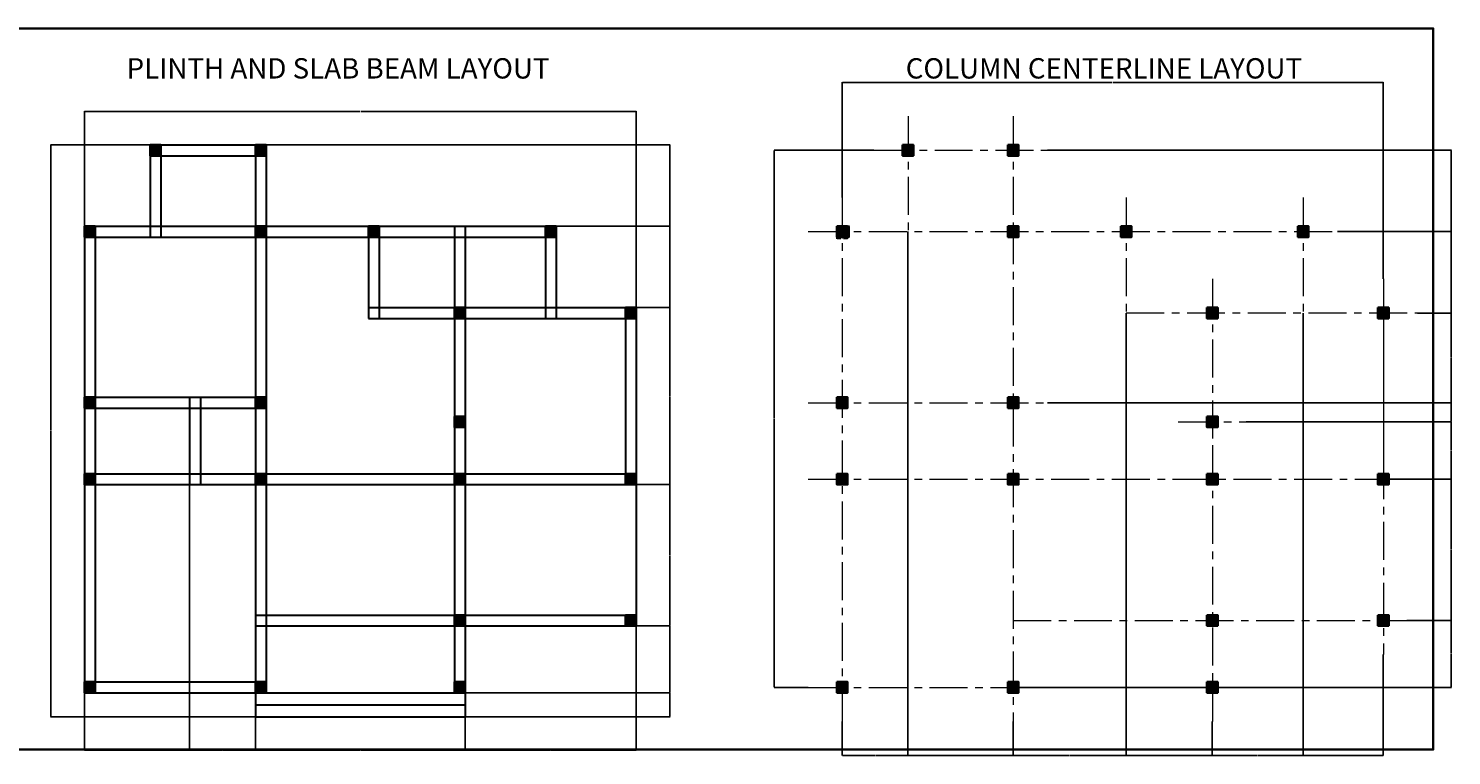
# Model space of a CAD drawing. Units: inches. Extents: x 1332 to 3175, y 1481 to 2088.
# Tile 5 of 5: x 1985 to 3175, y 1481 to 2088. Entities that reach past the tile are written whole.
import ezdxf

# ---------------------------------------------------------------- set-up
doc = ezdxf.new("R2010")
doc.units = ezdxf.units.IN
doc.linetypes.add('CENTER', pattern=[50.8, 31.75, -6.35, 6.35, -6.35])
for name, color, linetype, lineweight in [('A-ANNO-DIMS', 2, 'Continuous', 18), ('A-ANNO-TITL', 6, 'Continuous', 30), ('A-ANNO-TTLB', 7, 'Continuous', 35), ('S-BEAM', 7, 'Continuous', 30), ('S-COLS', 1, 'Continuous', 35), ('S-GRID', 8, 'CENTER', 18)]:
    doc.layers.add(name, color=color, linetype=linetype, lineweight=lineweight)
doc.styles.get("Standard").update_dxf_attribs({"font": 'arial.ttf'})
doc.dimstyles.get("Standard").update_dxf_attribs({"dimtxt": 0.18, "dimasz": 0.18, "dimexe": 0.18, "dimexo": 0.0625, "dimgap": 0.09, "dimtad": 0, "dimtih": 1, "dimtoh": 1, "dimdec": 4, "dimzin": 0, "dimdsep": 46, "dimtxsty": 'Standard', "dimcen": 0.09, "dimadec": 0, "dimazin": 0, "dimtfac": 1, "dimtdec": 4, "dimtofl": 0, "dimtmove": 0, "dimatfit": 3, "dimfxl": 1, "dimtolj": 1, "dimtzin": 0, "dimarcsym": 0})

# ---------------------------------------------------------------- blocks, each defined once
blk = doc.blocks.new('COL-SQUARE-9-STRUCT')
h = blk.add_hatch(color=256)
h.dxf.hatch_style = 1
h.paths.add_polyline_path([(9, 9), (0, 9), (0, 0), (9, 0)])
blk.add_lwpolyline([(0, 9), (9, 9), (9, 0), (0, 0)], close=True)
blk = doc.blocks.new('*D13')
at = {"layer": 'A-ANNO-DIMS', "color": 0, "lineweight": -2, "transparency": 16777216}
for p, q in [((2661, 1914.1), (2661, 1912.6)), ((2661.2, 1912.8), (2664.5, 1912.8)), ((2669.9, 1912.8), (2666.6, 1912.8)), ((2670, 1914.1), (2670, 1912.6))]:
    blk.add_line(p, q, dxfattribs=at)
at = {"layer": 'A-ANNO-DIMS', "color": 0, "transparency": 16777216}
for points in [[(2661.2, 1912.8), (2661.2, 1912.7), (2661, 1912.8)], [(2669.9, 1912.8), (2669.9, 1912.7), (2670, 1912.8)]]:
    blk.add_solid(points, dxfattribs=at)
at = {"layer": 'Defpoints', "color": 0, "transparency": 16777216}
for p in [(2661, 1914.1), (2670, 1914.1), (2670, 1912.8)]:
    blk.add_point(p, dxfattribs=at)
at = {"layer": 'A-ANNO-DIMS', "color": 0, "transparency": 16777216, "insert": (2665.5, 1912.8), "char_height": 0.18, "attachment_point": 5}
blk.add_mtext('\\A1;COLUMN 9 TYP.', dxfattribs=at)
blk = doc.blocks.new('*D14')
at = {"layer": 'A-ANNO-DIMS', "color": 0, "lineweight": -2, "transparency": 16777216}
for p, q in [((2670.1, 1923.1), (2671.6, 1923.1)), ((2671.4, 1922.9), (2671.4, 1918.8)), ((2671.4, 1914.3), (2671.4, 1918.4)), ((2670.1, 1914.1), (2671.6, 1914.1))]:
    blk.add_line(p, q, dxfattribs=at)
at = {"layer": 'A-ANNO-DIMS', "color": 0, "transparency": 16777216}
for points in [[(2671.4, 1922.9), (2671.4, 1922.9), (2671.4, 1923.1)], [(2671.4, 1914.3), (2671.4, 1914.3), (2671.4, 1914.1)]]:
    blk.add_solid(points, dxfattribs=at)
at = {"layer": 'Defpoints', "color": 0, "transparency": 16777216}
for p in [(2670, 1923.1), (2671.4, 1923.1), (2670, 1914.1)]:
    blk.add_point(p, dxfattribs=at)
at = {"layer": 'A-ANNO-DIMS', "color": 0, "transparency": 16777216, "insert": (2671.4, 1918.6), "char_height": 0.18, "attachment_point": 5}
blk.add_mtext('\\A1;9 TYP.', dxfattribs=at)
blk = doc.blocks.new('*D56')
at = {"layer": 'A-ANNO-DIMS', "color": 0, "lineweight": -2, "transparency": 16777216}
for p, q in [((2031.8, 1923.2), (2031.8, 2019.4)), ((2032, 2019.2), (2262.1, 2019.2)), ((2493.1, 2019.2), (2262.9, 2019.2)), ((2493.3, 1855.2), (2493.3, 2019.4))]:
    blk.add_line(p, q, dxfattribs=at)
at = {"layer": 'A-ANNO-DIMS', "color": 0, "transparency": 16777216}
for points in [[(2032, 2019.2), (2032, 2019.2), (2031.8, 2019.2)], [(2493.1, 2019.2), (2493.1, 2019.2), (2493.3, 2019.2)]]:
    blk.add_solid(points, dxfattribs=at)
at = {"layer": 'Defpoints', "color": 0, "transparency": 16777216}
for p in [(2493.3, 2019.2), (2031.8, 1923.1), (2493.3, 1855.1)]:
    blk.add_point(p, dxfattribs=at)
at = {"layer": 'A-ANNO-DIMS', "color": 0, "transparency": 16777216, "insert": (2262.5, 2019.2), "char_height": 0.18, "attachment_point": 5}
blk.add_mtext('\\A1;461.5', dxfattribs=at)
blk = doc.blocks.new('*D57')
at = {"layer": 'A-ANNO-DIMS', "color": 0, "lineweight": -2, "transparency": 16777216}
for p, q in [((2086.7, 1991.1), (2003.5, 1991.1)), ((2003.7, 1990.9), (2003.7, 1752.3)), ((2003.7, 1513.3), (2003.7, 1751.9)), ((2174.7, 1513.1), (2003.5, 1513.1))]:
    blk.add_line(p, q, dxfattribs=at)
at = {"layer": 'A-ANNO-DIMS', "color": 0, "transparency": 16777216}
for points in [[(2003.7, 1990.9), (2003.7, 1990.9), (2003.7, 1991.1)], [(2003.7, 1513.3), (2003.7, 1513.3), (2003.7, 1513.1)]]:
    blk.add_solid(points, dxfattribs=at)
at = {"layer": 'Defpoints', "color": 0, "transparency": 16777216}
for p in [(2003.7, 1991.1), (2086.8, 1991.1), (2174.8, 1513.1)]:
    blk.add_point(p, dxfattribs=at)
at = {"layer": 'A-ANNO-DIMS', "color": 0, "transparency": 16777216, "insert": (2003.7, 1752.1), "char_height": 0.18, "attachment_point": 5}
blk.add_mtext('\\A1;478', dxfattribs=at)
blk = doc.blocks.new('*D58')
at = {"layer": 'A-ANNO-DIMS', "color": 0, "lineweight": -2, "transparency": 16777216}
for p, q in [((2119.8, 1707.1), (2119.8, 1484.8)), ((2031.8, 1533.1), (2031.8, 1484.8)), ((2032, 1485), (2075.6, 1485)), ((2119.6, 1485), (2076, 1485))]:
    blk.add_line(p, q, dxfattribs=at)
at = {"layer": 'A-ANNO-DIMS', "color": 0, "transparency": 16777216}
for points in [[(2032, 1485), (2032, 1485), (2031.8, 1485)], [(2119.6, 1485), (2119.6, 1485), (2119.8, 1485)]]:
    blk.add_solid(points, dxfattribs=at)
at = {"layer": 'Defpoints', "color": 0, "transparency": 16777216}
for p in [(2119.8, 1707.1), (2031.8, 1533.1), (2119.8, 1485)]:
    blk.add_point(p, dxfattribs=at)
at = {"layer": 'A-ANNO-DIMS', "color": 0, "transparency": 16777216, "insert": (2075.8, 1485), "char_height": 0.18, "attachment_point": 5}
blk.add_mtext('\\A1;88', dxfattribs=at)
blk = doc.blocks.new('*D59')
at = {"layer": 'A-ANNO-DIMS', "color": 0, "lineweight": -2, "transparency": 16777216}
for p, q in [((2119.8, 1707.1), (2119.8, 1484.8)), ((2174.8, 1513.1), (2174.8, 1484.8)), ((2120, 1485), (2147.1, 1485)), ((2174.6, 1485), (2147.5, 1485))]:
    blk.add_line(p, q, dxfattribs=at)
at = {"layer": 'A-ANNO-DIMS', "color": 0, "transparency": 16777216}
for points in [[(2120, 1485), (2120, 1485), (2119.8, 1485)], [(2174.6, 1485), (2174.6, 1485), (2174.8, 1485)]]:
    blk.add_solid(points, dxfattribs=at)
at = {"layer": 'Defpoints', "color": 0, "transparency": 16777216}
for p in [(2119.8, 1707.1), (2174.8, 1513.1), (2174.8, 1485)]:
    blk.add_point(p, dxfattribs=at)
at = {"layer": 'A-ANNO-DIMS', "color": 0, "transparency": 16777216, "insert": (2147.3, 1485), "char_height": 0.18, "attachment_point": 5}
blk.add_mtext('\\A1;55', dxfattribs=at)
blk = doc.blocks.new('*D60')
at = {"layer": 'A-ANNO-DIMS', "color": 0, "lineweight": -2, "transparency": 16777216}
for p, q in [((2174.8, 1513.1), (2174.8, 1484.8)), ((2350.3, 1513.1), (2350.3, 1484.8)), ((2175, 1485), (2262.1, 1485)), ((2350.1, 1485), (2262.9, 1485))]:
    blk.add_line(p, q, dxfattribs=at)
at = {"layer": 'A-ANNO-DIMS', "color": 0, "transparency": 16777216}
for points in [[(2175, 1485), (2175, 1485), (2174.8, 1485)], [(2350.1, 1485), (2350.1, 1485), (2350.3, 1485)]]:
    blk.add_solid(points, dxfattribs=at)
at = {"layer": 'Defpoints', "color": 0, "transparency": 16777216}
for p in [(2174.8, 1513.1), (2350.3, 1513.1), (2350.3, 1485)]:
    blk.add_point(p, dxfattribs=at)
at = {"layer": 'A-ANNO-DIMS', "color": 0, "transparency": 16777216, "insert": (2262.5, 1485), "char_height": 0.18, "attachment_point": 5}
blk.add_mtext('\\A1;175.5', dxfattribs=at)
blk = doc.blocks.new('*D61')
at = {"layer": 'A-ANNO-DIMS', "color": 0, "lineweight": -2, "transparency": 16777216}
for p, q in [((2493.3, 1589.1), (2493.3, 1484.8)), ((2350.3, 1513.1), (2350.3, 1484.8)), ((2350.5, 1485), (2421.5, 1485)), ((2493.1, 1485), (2422.1, 1485))]:
    blk.add_line(p, q, dxfattribs=at)
at = {"layer": 'A-ANNO-DIMS', "color": 0, "transparency": 16777216}
for points in [[(2350.5, 1485), (2350.5, 1485), (2350.3, 1485)], [(2493.1, 1485), (2493.1, 1485), (2493.3, 1485)]]:
    blk.add_solid(points, dxfattribs=at)
at = {"layer": 'Defpoints', "color": 0, "transparency": 16777216}
for p in [(2493.3, 1589.1), (2350.3, 1513.1), (2493.3, 1485)]:
    blk.add_point(p, dxfattribs=at)
at = {"layer": 'A-ANNO-DIMS', "color": 0, "transparency": 16777216, "insert": (2421.8, 1485), "char_height": 0.18, "attachment_point": 5}
blk.add_mtext('\\A1;143', dxfattribs=at)
blk = doc.blocks.new('*D62')
at = {"layer": 'A-ANNO-DIMS', "color": 0, "lineweight": -2, "transparency": 16777216}
for p, q in [((2350.3, 1533.1), (2521.6, 1533.1)), ((2521.4, 1532.9), (2521.4, 1523.3)), ((2350.3, 1513.1), (2521.6, 1513.1)), ((2521.4, 1513.3), (2521.4, 1522.9))]:
    blk.add_line(p, q, dxfattribs=at)
at = {"layer": 'A-ANNO-DIMS', "color": 0, "transparency": 16777216}
for points in [[(2521.4, 1532.9), (2521.4, 1532.9), (2521.4, 1533.1)], [(2521.4, 1513.3), (2521.4, 1513.3), (2521.4, 1513.1)]]:
    blk.add_solid(points, dxfattribs=at)
at = {"layer": 'Defpoints', "color": 0, "transparency": 16777216}
for p in [(2350.3, 1533.1), (2521.4, 1533.1), (2350.3, 1513.1)]:
    blk.add_point(p, dxfattribs=at)
at = {"layer": 'A-ANNO-DIMS', "color": 0, "transparency": 16777216, "insert": (2521.4, 1523.1), "char_height": 0.18, "attachment_point": 5}
blk.add_mtext('\\A1;20', dxfattribs=at)
blk = doc.blocks.new('*D63')
at = {"layer": 'A-ANNO-DIMS', "color": 0, "lineweight": -2, "transparency": 16777216}
for p, q in [((2493.3, 1589.1), (2521.6, 1589.1)), ((2521.4, 1588.9), (2521.4, 1561.3)), ((2521.4, 1533.3), (2521.4, 1560.9)), ((2350.3, 1533.1), (2521.6, 1533.1))]:
    blk.add_line(p, q, dxfattribs=at)
at = {"layer": 'A-ANNO-DIMS', "color": 0, "transparency": 16777216}
for points in [[(2521.4, 1588.9), (2521.4, 1588.9), (2521.4, 1589.1)], [(2521.4, 1533.3), (2521.4, 1533.3), (2521.4, 1533.1)]]:
    blk.add_solid(points, dxfattribs=at)
at = {"layer": 'Defpoints', "color": 0, "transparency": 16777216}
for p in [(2493.3, 1589.1), (2521.4, 1589.1), (2350.3, 1533.1)]:
    blk.add_point(p, dxfattribs=at)
at = {"layer": 'A-ANNO-DIMS', "color": 0, "transparency": 16777216, "insert": (2521.4, 1561.1), "char_height": 0.18, "attachment_point": 5}
blk.add_mtext('\\A1;56', dxfattribs=at)
blk = doc.blocks.new('*D64')
at = {"layer": 'A-ANNO-DIMS', "color": 0, "lineweight": -2, "transparency": 16777216}
for p, q in [((2493.3, 1707.1), (2521.6, 1707.1)), ((2521.4, 1706.9), (2521.4, 1648.3)), ((2521.4, 1589.3), (2521.4, 1647.9)), ((2493.3, 1589.1), (2521.6, 1589.1))]:
    blk.add_line(p, q, dxfattribs=at)
at = {"layer": 'A-ANNO-DIMS', "color": 0, "transparency": 16777216}
for points in [[(2521.4, 1706.9), (2521.4, 1706.9), (2521.4, 1707.1)], [(2521.4, 1589.3), (2521.4, 1589.3), (2521.4, 1589.1)]]:
    blk.add_solid(points, dxfattribs=at)
at = {"layer": 'Defpoints', "color": 0, "transparency": 16777216}
for p in [(2493.3, 1707.1), (2521.4, 1707.1), (2493.3, 1589.1)]:
    blk.add_point(p, dxfattribs=at)
at = {"layer": 'A-ANNO-DIMS', "color": 0, "transparency": 16777216, "insert": (2521.4, 1648.1), "char_height": 0.18, "attachment_point": 5}
blk.add_mtext('\\A1;118', dxfattribs=at)
blk = doc.blocks.new('*D65')
at = {"layer": 'A-ANNO-DIMS', "color": 0, "lineweight": -2, "transparency": 16777216}
for p, q in [((2493.3, 1855.1), (2521.6, 1855.1)), ((2521.4, 1854.9), (2521.4, 1781.3)), ((2521.4, 1707.3), (2521.4, 1780.9)), ((2493.3, 1707.1), (2521.6, 1707.1))]:
    blk.add_line(p, q, dxfattribs=at)
at = {"layer": 'A-ANNO-DIMS', "color": 0, "transparency": 16777216}
for points in [[(2521.4, 1854.9), (2521.4, 1854.9), (2521.4, 1855.1)], [(2521.4, 1707.3), (2521.4, 1707.3), (2521.4, 1707.1)]]:
    blk.add_solid(points, dxfattribs=at)
at = {"layer": 'Defpoints', "color": 0, "transparency": 16777216}
for p in [(2493.3, 1855.1), (2521.4, 1855.1), (2493.3, 1707.1)]:
    blk.add_point(p, dxfattribs=at)
at = {"layer": 'A-ANNO-DIMS', "color": 0, "transparency": 16777216, "insert": (2521.4, 1781.1), "char_height": 0.18, "attachment_point": 5}
blk.add_mtext('\\A1;148', dxfattribs=at)
blk = doc.blocks.new('*D66')
at = {"layer": 'A-ANNO-DIMS', "color": 0, "lineweight": -2, "transparency": 16777216}
for p, q in [((2426.3, 1923.1), (2521.6, 1923.1)), ((2521.4, 1922.9), (2521.4, 1889.3)), ((2521.4, 1855.3), (2521.4, 1888.9)), ((2493.3, 1855.1), (2521.6, 1855.1))]:
    blk.add_line(p, q, dxfattribs=at)
at = {"layer": 'A-ANNO-DIMS', "color": 0, "transparency": 16777216}
for points in [[(2521.4, 1922.9), (2521.4, 1922.9), (2521.4, 1923.1)], [(2521.4, 1855.3), (2521.4, 1855.3), (2521.4, 1855.1)]]:
    blk.add_solid(points, dxfattribs=at)
at = {"layer": 'Defpoints', "color": 0, "transparency": 16777216}
for p in [(2426.3, 1923.1), (2521.4, 1923.1), (2493.3, 1855.1)]:
    blk.add_point(p, dxfattribs=at)
at = {"layer": 'A-ANNO-DIMS', "color": 0, "transparency": 16777216, "insert": (2521.4, 1889.1), "char_height": 0.18, "attachment_point": 5}
blk.add_mtext('\\A1;68', dxfattribs=at)
blk = doc.blocks.new('*D67')
at = {"layer": 'A-ANNO-DIMS', "color": 0, "lineweight": -2, "transparency": 16777216}
for p, q in [((2183.8, 1991.1), (2521.6, 1991.1)), ((2521.4, 1990.9), (2521.4, 1957.3)), ((2521.4, 1923.3), (2521.4, 1956.9)), ((2426.3, 1923.1), (2521.6, 1923.1))]:
    blk.add_line(p, q, dxfattribs=at)
at = {"layer": 'A-ANNO-DIMS', "color": 0, "transparency": 16777216}
for points in [[(2521.4, 1990.9), (2521.4, 1990.9), (2521.4, 1991.1)], [(2521.4, 1923.3), (2521.4, 1923.3), (2521.4, 1923.1)]]:
    blk.add_solid(points, dxfattribs=at)
at = {"layer": 'Defpoints', "color": 0, "transparency": 16777216}
for p in [(2183.8, 1991.1), (2521.4, 1991.1), (2426.3, 1923.1)]:
    blk.add_point(p, dxfattribs=at)
at = {"layer": 'A-ANNO-DIMS', "color": 0, "transparency": 16777216, "insert": (2521.4, 1957.1), "char_height": 0.18, "attachment_point": 5}
blk.add_mtext('\\A1;68', dxfattribs=at)
blk = doc.blocks.new('*D68')
at = {"layer": 'A-ANNO-DIMS', "color": 0, "lineweight": -2, "transparency": 16777216}
for p, q in [((2665.5, 1947.2), (2665.5, 2043.6)), ((2665.7, 2043.4), (2891.4, 2043.4)), ((3117.9, 2043.4), (2892.2, 2043.4)), ((3118, 1879.2), (3118, 2043.6))]:
    blk.add_line(p, q, dxfattribs=at)
at = {"layer": 'A-ANNO-DIMS', "color": 0, "transparency": 16777216}
for points in [[(2665.7, 2043.4), (2665.7, 2043.4), (2665.5, 2043.4)], [(3117.9, 2043.4), (3117.9, 2043.4), (3118, 2043.4)]]:
    blk.add_solid(points, dxfattribs=at)
at = {"layer": 'Defpoints', "color": 0, "transparency": 16777216}
for p in [(3118, 2043.4), (2665.5, 1947.1), (3118, 1879.1)]:
    blk.add_point(p, dxfattribs=at)
at = {"layer": 'A-ANNO-DIMS', "color": 0, "transparency": 16777216, "insert": (2891.8, 2043.4), "char_height": 0.18, "attachment_point": 5}
blk.add_mtext('\\A1;452.5', dxfattribs=at)
blk = doc.blocks.new('*D69')
at = {"layer": 'A-ANNO-DIMS', "color": 0, "lineweight": -2, "transparency": 16777216}
for p, q in [((2692, 1986.6), (2608.6, 1986.6)), ((2608.7, 1986.4), (2608.7, 1762.3)), ((2608.7, 1537.8), (2608.7, 1761.9)), ((2637, 1537.6), (2608.6, 1537.6))]:
    blk.add_line(p, q, dxfattribs=at)
at = {"layer": 'A-ANNO-DIMS', "color": 0, "transparency": 16777216}
for points in [[(2608.7, 1986.4), (2608.8, 1986.4), (2608.7, 1986.6)], [(2608.7, 1537.8), (2608.8, 1537.8), (2608.7, 1537.6)]]:
    blk.add_solid(points, dxfattribs=at)
at = {"layer": 'Defpoints', "color": 0, "transparency": 16777216}
for p in [(2608.7, 1986.6), (2692, 1986.6), (2637, 1537.6)]:
    blk.add_point(p, dxfattribs=at)
at = {"layer": 'A-ANNO-DIMS', "color": 0, "transparency": 16777216, "insert": (2608.7, 1762.1), "char_height": 0.18, "attachment_point": 5}
blk.add_mtext('\\A1;449', dxfattribs=at)
blk = doc.blocks.new('*D70')
at = {"layer": 'A-ANNO-DIMS', "color": 0, "lineweight": -2, "transparency": 16777216}
for p, q in [((2720.5, 1918.6), (2720.5, 1480.6)), ((2665.5, 1509.1), (2665.5, 1480.6)), ((2665.7, 1480.8), (2692.8, 1480.8)), ((2720.4, 1480.8), (2693.3, 1480.8))]:
    blk.add_line(p, q, dxfattribs=at)
at = {"layer": 'A-ANNO-DIMS', "color": 0, "transparency": 16777216}
for points in [[(2665.7, 1480.8), (2665.7, 1480.8), (2665.5, 1480.8)], [(2720.4, 1480.8), (2720.4, 1480.8), (2720.5, 1480.8)]]:
    blk.add_solid(points, dxfattribs=at)
at = {"layer": 'Defpoints', "color": 0, "transparency": 16777216}
for p in [(2720.5, 1918.6), (2665.5, 1509.1), (2720.5, 1480.8)]:
    blk.add_point(p, dxfattribs=at)
at = {"layer": 'A-ANNO-DIMS', "color": 0, "transparency": 16777216, "insert": (2693, 1480.8), "char_height": 0.18, "attachment_point": 5}
blk.add_mtext('\\A1;55', dxfattribs=at)
blk = doc.blocks.new('*D71')
at = {"layer": 'A-ANNO-DIMS', "color": 0, "lineweight": -2, "transparency": 16777216}
for p, q in [((2720.5, 1918.6), (2720.5, 1480.6)), ((2808.5, 1509.1), (2808.5, 1480.6)), ((2720.7, 1480.8), (2764.3, 1480.8)), ((2808.4, 1480.8), (2764.8, 1480.8))]:
    blk.add_line(p, q, dxfattribs=at)
at = {"layer": 'A-ANNO-DIMS', "color": 0, "transparency": 16777216}
for points in [[(2720.7, 1480.8), (2720.7, 1480.8), (2720.5, 1480.8)], [(2808.4, 1480.8), (2808.4, 1480.8), (2808.5, 1480.8)]]:
    blk.add_solid(points, dxfattribs=at)
at = {"layer": 'Defpoints', "color": 0, "transparency": 16777216}
for p in [(2720.5, 1918.6), (2808.5, 1509.1), (2808.5, 1480.8)]:
    blk.add_point(p, dxfattribs=at)
at = {"layer": 'A-ANNO-DIMS', "color": 0, "transparency": 16777216, "insert": (2764.5, 1480.8), "char_height": 0.18, "attachment_point": 5}
blk.add_mtext('\\A1;88', dxfattribs=at)
blk = doc.blocks.new('*D72')
at = {"layer": 'A-ANNO-DIMS', "color": 0, "lineweight": -2, "transparency": 16777216}
for p, q in [((2903, 1850.6), (2903, 1480.6)), ((2808.5, 1509.1), (2808.5, 1480.6)), ((2808.7, 1480.8), (2855.5, 1480.8)), ((2902.9, 1480.8), (2856.1, 1480.8))]:
    blk.add_line(p, q, dxfattribs=at)
at = {"layer": 'A-ANNO-DIMS', "color": 0, "transparency": 16777216}
for points in [[(2808.7, 1480.8), (2808.7, 1480.8), (2808.5, 1480.8)], [(2902.9, 1480.8), (2902.9, 1480.8), (2903, 1480.8)]]:
    blk.add_solid(points, dxfattribs=at)
at = {"layer": 'Defpoints', "color": 0, "transparency": 16777216}
for p in [(2903, 1850.6), (2808.5, 1509.1), (2903, 1480.8)]:
    blk.add_point(p, dxfattribs=at)
at = {"layer": 'A-ANNO-DIMS', "color": 0, "transparency": 16777216, "insert": (2855.8, 1480.8), "char_height": 0.18, "attachment_point": 5}
blk.add_mtext('\\A1;94.5', dxfattribs=at)
blk = doc.blocks.new('*D73')
at = {"layer": 'A-ANNO-DIMS', "color": 0, "lineweight": -2, "transparency": 16777216}
for p, q in [((2903, 1850.6), (2903, 1480.6)), ((2975, 1509.1), (2975, 1480.6)), ((2903.2, 1480.8), (2938.8, 1480.8)), ((2974.9, 1480.8), (2939.3, 1480.8))]:
    blk.add_line(p, q, dxfattribs=at)
at = {"layer": 'A-ANNO-DIMS', "color": 0, "transparency": 16777216}
for points in [[(2903.2, 1480.8), (2903.2, 1480.8), (2903, 1480.8)], [(2974.9, 1480.8), (2974.9, 1480.8), (2975, 1480.8)]]:
    blk.add_solid(points, dxfattribs=at)
at = {"layer": 'Defpoints', "color": 0, "transparency": 16777216}
for p in [(2903, 1850.6), (2975, 1509.1), (2975, 1480.8)]:
    blk.add_point(p, dxfattribs=at)
at = {"layer": 'A-ANNO-DIMS', "color": 0, "transparency": 16777216, "insert": (2939, 1480.8), "char_height": 0.18, "attachment_point": 5}
blk.add_mtext('\\A1;72', dxfattribs=at)
blk = doc.blocks.new('*D74')
at = {"layer": 'A-ANNO-DIMS', "color": 0, "lineweight": -2, "transparency": 16777216}
for p, q in [((3051, 1850.6), (3051, 1480.6)), ((2975, 1509.1), (2975, 1480.6)), ((2975.2, 1480.8), (3012.8, 1480.8)), ((3050.9, 1480.8), (3013.3, 1480.8))]:
    blk.add_line(p, q, dxfattribs=at)
at = {"layer": 'A-ANNO-DIMS', "color": 0, "transparency": 16777216}
for points in [[(2975.2, 1480.8), (2975.2, 1480.8), (2975, 1480.8)], [(3050.9, 1480.8), (3050.9, 1480.8), (3051, 1480.8)]]:
    blk.add_solid(points, dxfattribs=at)
at = {"layer": 'Defpoints', "color": 0, "transparency": 16777216}
for p in [(3051, 1850.6), (2975, 1509.1), (3051, 1480.8)]:
    blk.add_point(p, dxfattribs=at)
at = {"layer": 'A-ANNO-DIMS', "color": 0, "transparency": 16777216, "insert": (3013, 1480.8), "char_height": 0.18, "attachment_point": 5}
blk.add_mtext('\\A1;76', dxfattribs=at)
blk = doc.blocks.new('*D75')
at = {"layer": 'A-ANNO-DIMS', "color": 0, "lineweight": -2, "transparency": 16777216}
for p, q in [((3051, 1850.6), (3051, 1480.6)), ((3118, 1565.1), (3118, 1480.6)), ((3051.2, 1480.8), (3084.3, 1480.8)), ((3117.9, 1480.8), (3084.8, 1480.8))]:
    blk.add_line(p, q, dxfattribs=at)
at = {"layer": 'A-ANNO-DIMS', "color": 0, "transparency": 16777216}
for points in [[(3051.2, 1480.8), (3051.2, 1480.8), (3051, 1480.8)], [(3117.9, 1480.8), (3117.9, 1480.8), (3118, 1480.8)]]:
    blk.add_solid(points, dxfattribs=at)
at = {"layer": 'Defpoints', "color": 0, "transparency": 16777216}
for p in [(3051, 1850.6), (3118, 1565.1), (3118, 1480.8)]:
    blk.add_point(p, dxfattribs=at)
at = {"layer": 'A-ANNO-DIMS', "color": 0, "transparency": 16777216, "insert": (3084.5, 1480.8), "char_height": 0.18, "attachment_point": 5}
blk.add_mtext('\\A1;67', dxfattribs=at)
blk = doc.blocks.new('*D76')
at = {"layer": 'A-ANNO-DIMS', "color": 0, "lineweight": -2, "transparency": 16777216}
for p, q in [((3137.6, 1593.6), (3175, 1593.6)), ((3174.8, 1593.4), (3174.8, 1565.8)), ((3174.8, 1537.8), (3174.8, 1565.4)), ((2813.1, 1537.6), (3175, 1537.6))]:
    blk.add_line(p, q, dxfattribs=at)
at = {"layer": 'A-ANNO-DIMS', "color": 0, "transparency": 16777216}
for points in [[(3174.8, 1593.4), (3174.9, 1593.4), (3174.8, 1593.6)], [(3174.8, 1537.8), (3174.9, 1537.8), (3174.8, 1537.6)]]:
    blk.add_solid(points, dxfattribs=at)
at = {"layer": 'Defpoints', "color": 0, "transparency": 16777216}
for p in [(3137.5, 1593.6), (3174.8, 1593.6), (2813, 1537.6)]:
    blk.add_point(p, dxfattribs=at)
at = {"layer": 'A-ANNO-DIMS', "color": 0, "transparency": 16777216, "insert": (3174.8, 1565.6), "char_height": 0.18, "attachment_point": 5}
blk.add_mtext('\\A1;56', dxfattribs=at)
blk = doc.blocks.new('*D77')
at = {"layer": 'A-ANNO-DIMS', "color": 0, "lineweight": -2, "transparency": 16777216}
for p, q in [((3122.6, 1711.6), (3175, 1711.6)), ((3174.8, 1711.4), (3174.8, 1652.8)), ((3174.8, 1593.8), (3174.8, 1652.4)), ((3137.6, 1593.6), (3175, 1593.6))]:
    blk.add_line(p, q, dxfattribs=at)
at = {"layer": 'A-ANNO-DIMS', "color": 0, "transparency": 16777216}
for points in [[(3174.8, 1711.4), (3174.9, 1711.4), (3174.8, 1711.6)], [(3174.8, 1593.8), (3174.9, 1593.8), (3174.8, 1593.6)]]:
    blk.add_solid(points, dxfattribs=at)
at = {"layer": 'Defpoints', "color": 0, "transparency": 16777216}
for p in [(3122.5, 1711.6), (3174.8, 1711.6), (3137.5, 1593.6)]:
    blk.add_point(p, dxfattribs=at)
at = {"layer": 'A-ANNO-DIMS', "color": 0, "transparency": 16777216, "insert": (3174.8, 1652.6), "char_height": 0.18, "attachment_point": 5}
blk.add_mtext('\\A1;118', dxfattribs=at)
blk = doc.blocks.new('*D78')
at = {"layer": 'A-ANNO-DIMS', "color": 0, "lineweight": -2, "transparency": 16777216}
for p, q in [((3003.4, 1759.6), (3175, 1759.6)), ((3174.8, 1759.4), (3174.8, 1735.8)), ((3174.8, 1711.8), (3174.8, 1735.4)), ((3122.6, 1711.6), (3175, 1711.6))]:
    blk.add_line(p, q, dxfattribs=at)
at = {"layer": 'A-ANNO-DIMS', "color": 0, "transparency": 16777216}
for points in [[(3174.8, 1759.4), (3174.9, 1759.4), (3174.8, 1759.6)], [(3174.8, 1711.8), (3174.9, 1711.8), (3174.8, 1711.6)]]:
    blk.add_solid(points, dxfattribs=at)
at = {"layer": 'Defpoints', "color": 0, "transparency": 16777216}
for p in [(3003.3, 1759.6), (3174.8, 1759.6), (3122.5, 1711.6)]:
    blk.add_point(p, dxfattribs=at)
at = {"layer": 'A-ANNO-DIMS', "color": 0, "transparency": 16777216, "insert": (3174.8, 1735.6), "char_height": 0.18, "attachment_point": 5}
blk.add_mtext('\\A1;48', dxfattribs=at)
blk = doc.blocks.new('*D79')
at = {"layer": 'A-ANNO-DIMS', "color": 0, "lineweight": -2, "transparency": 16777216}
for p, q in [((2837.1, 1775.6), (3175, 1775.6)), ((3174.8, 1775.4), (3174.8, 1767.8)), ((3174.8, 1759.8), (3174.8, 1767.4)), ((3003.4, 1759.6), (3175, 1759.6))]:
    blk.add_line(p, q, dxfattribs=at)
at = {"layer": 'A-ANNO-DIMS', "color": 0, "transparency": 16777216}
for points in [[(3174.8, 1775.4), (3174.9, 1775.4), (3174.8, 1775.6)], [(3174.8, 1759.8), (3174.9, 1759.8), (3174.8, 1759.6)]]:
    blk.add_solid(points, dxfattribs=at)
at = {"layer": 'Defpoints', "color": 0, "transparency": 16777216}
for p in [(2837, 1775.6), (3174.8, 1775.6), (3003.3, 1759.6)]:
    blk.add_point(p, dxfattribs=at)
at = {"layer": 'A-ANNO-DIMS', "color": 0, "transparency": 16777216, "insert": (3174.8, 1767.6), "char_height": 0.18, "attachment_point": 5}
blk.add_mtext('\\A1;16', dxfattribs=at)
blk = doc.blocks.new('*D80')
at = {"layer": 'A-ANNO-DIMS', "color": 0, "lineweight": -2, "transparency": 16777216}
for p, q in [((3146.6, 1850.6), (3175, 1850.6)), ((3174.8, 1850.4), (3174.8, 1813.3)), ((3174.8, 1775.8), (3174.8, 1812.9)), ((2837.1, 1775.6), (3175, 1775.6))]:
    blk.add_line(p, q, dxfattribs=at)
at = {"layer": 'A-ANNO-DIMS', "color": 0, "transparency": 16777216}
for points in [[(3174.8, 1850.4), (3174.9, 1850.4), (3174.8, 1850.6)], [(3174.8, 1775.8), (3174.9, 1775.8), (3174.8, 1775.6)]]:
    blk.add_solid(points, dxfattribs=at)
at = {"layer": 'Defpoints', "color": 0, "transparency": 16777216}
for p in [(3146.5, 1850.6), (3174.8, 1850.6), (2837, 1775.6)]:
    blk.add_point(p, dxfattribs=at)
at = {"layer": 'A-ANNO-DIMS', "color": 0, "transparency": 16777216, "insert": (3174.8, 1813.1), "char_height": 0.18, "attachment_point": 5}
blk.add_mtext('\\A1;75', dxfattribs=at)
blk = doc.blocks.new('*D81')
at = {"layer": 'A-ANNO-DIMS', "color": 0, "lineweight": -2, "transparency": 16777216}
for p, q in [((3079.6, 1918.6), (3175, 1918.6)), ((3174.8, 1918.4), (3174.8, 1884.8)), ((3174.8, 1850.8), (3174.8, 1884.4)), ((3146.6, 1850.6), (3175, 1850.6))]:
    blk.add_line(p, q, dxfattribs=at)
at = {"layer": 'A-ANNO-DIMS', "color": 0, "transparency": 16777216}
for points in [[(3174.8, 1918.4), (3174.9, 1918.4), (3174.8, 1918.6)], [(3174.8, 1850.8), (3174.9, 1850.8), (3174.8, 1850.6)]]:
    blk.add_solid(points, dxfattribs=at)
at = {"layer": 'Defpoints', "color": 0, "transparency": 16777216}
for p in [(3079.5, 1918.6), (3174.8, 1918.6), (3146.5, 1850.6)]:
    blk.add_point(p, dxfattribs=at)
at = {"layer": 'A-ANNO-DIMS', "color": 0, "transparency": 16777216, "insert": (3174.8, 1884.6), "char_height": 0.18, "attachment_point": 5}
blk.add_mtext('\\A1;68', dxfattribs=at)
blk = doc.blocks.new('*D82')
at = {"layer": 'A-ANNO-DIMS', "color": 0, "lineweight": -2, "transparency": 16777216}
for p, q in [((2837.1, 1986.6), (3175, 1986.6)), ((3174.8, 1986.4), (3174.8, 1952.8)), ((3174.8, 1918.8), (3174.8, 1952.4)), ((3079.6, 1918.6), (3175, 1918.6))]:
    blk.add_line(p, q, dxfattribs=at)
at = {"layer": 'A-ANNO-DIMS', "color": 0, "transparency": 16777216}
for points in [[(3174.8, 1986.4), (3174.9, 1986.4), (3174.8, 1986.6)], [(3174.8, 1918.8), (3174.9, 1918.8), (3174.8, 1918.6)]]:
    blk.add_solid(points, dxfattribs=at)
at = {"layer": 'Defpoints', "color": 0, "transparency": 16777216}
for p in [(2837, 1986.6), (3174.8, 1986.6), (3079.5, 1918.6)]:
    blk.add_point(p, dxfattribs=at)
at = {"layer": 'A-ANNO-DIMS', "color": 0, "transparency": 16777216, "insert": (3174.8, 1952.6), "char_height": 0.18, "attachment_point": 5}
blk.add_mtext('\\A1;68', dxfattribs=at)

msp = doc.modelspace()

# ---------------------------------------------------------------- linework, layer by layer
at = {"layer": 'A-ANNO-TTLB'}
msp.add_lwpolyline([(1332.1674, 2088.4777), (3159.6908, 2088.4777), (3159.6908, 1485.6439), (1332.1674, 1485.6439)], close=True, dxfattribs=at)
at = {"layer": 'S-BEAM'}
for p, q in [((2086.7802, 1991.1183), (2086.7802, 1914.1183)), ((2086.7802, 1991.1183), (2183.7802, 1991.1183)), ((2086.7802, 1991.1183), (2183.7802, 1991.1183)), ((2095.7802, 1991.1183), (2095.7802, 1914.1183)), ((2174.7802, 1991.1183), (2174.7802, 1927.1183)), ((2174.7802, 1991.1183), (2174.7802, 1927.1183)), ((2183.7802, 1991.1183), (2183.7802, 1923.1183)), ((2183.7802, 1991.1183), (2183.7802, 1923.1183)), ((2086.7802, 1982.1183), (2183.7802, 1982.1183)), ((2086.7802, 1982.1183), (2183.7802, 1982.1183)), ((2031.7802, 1923.1183), (2426.2802, 1923.1183)), ((2031.7802, 1923.1183), (2426.2802, 1923.1183)), ((2031.7802, 1923.1183), (2031.7802, 1533.1183)), ((2031.7802, 1923.1183), (2031.7802, 1533.1183)), ((2040.7802, 1923.1183), (2040.7802, 1533.1183)), ((2040.7802, 1923.1183), (2040.7802, 1533.1183)), ((2174.7802, 1927.1183), (2174.7802, 1533.1183)), ((2174.7802, 1927.1183), (2174.7802, 1513.1183)), ((2174.7802, 1918.1183), (2174.7802, 1780.1183)), ((2174.7802, 1918.1183), (2174.7802, 1780.1183)), ((2183.7802, 1923.1183), (2183.7802, 1533.1183)), ((2183.7802, 1923.1183), (2183.7802, 1533.1183)), ((2269.2802, 1923.1183), (2269.2802, 1846.1183)), ((2269.2802, 1923.1183), (2269.2802, 1846.1183)), ((2278.2802, 1923.1183), (2278.2802, 1846.1183)), ((2278.2802, 1923.1183), (2278.2802, 1846.1183)), ((2341.2802, 1923.1183), (2341.2802, 1846.1183)), ((2341.2802, 1923.1183), (2341.2802, 1716.1183)), ((2350.2802, 1923.1183), (2350.2802, 1846.1183)), ((2350.2802, 1923.1183), (2350.2802, 1716.1183)), ((2417.2802, 1923.1183), (2417.2802, 1846.1183)), ((2417.2802, 1923.1183), (2417.2802, 1846.1183)), ((2426.2802, 1923.1183), (2426.2802, 1846.1183)), ((2426.2802, 1923.1183), (2426.2802, 1846.1183)), ((2031.7802, 1914.1183), (2426.2802, 1914.1183)), ((2031.7802, 1914.1183), (2426.2802, 1914.1183)), ((2269.2802, 1855.1183), (2493.2802, 1855.1183)), ((2269.2802, 1855.1183), (2493.2802, 1855.1183)), ((2269.2802, 1846.1183), (2493.2802, 1846.1183)), ((2269.2802, 1846.1183), (2493.2802, 1846.1183)), ((2484.2802, 1855.1183), (2484.2802, 1707.1183)), ((2484.2802, 1855.1183), (2484.2802, 1707.1183)), ((2493.2802, 1855.1183), (2493.2802, 1589.1183)), ((2493.2802, 1855.1183), (2493.2802, 1589.1183)), ((2031.7802, 1780.1183), (2174.7802, 1780.1183)), ((2031.7802, 1780.1183), (2183.7802, 1780.1183)), ((2119.7802, 1780.1183), (2119.7802, 1707.1183)), ((2128.7802, 1780.1183), (2128.7802, 1707.1183)), ((2031.7802, 1771.1183), (2174.7802, 1771.1183)), ((2031.7802, 1771.1183), (2183.7802, 1771.1183)), ((2031.7802, 1716.1183), (2493.2802, 1716.1183)), ((2031.7802, 1716.1183), (2493.2802, 1716.1183)), ((2040.7802, 1716.1183), (2174.7802, 1716.1183)), ((2040.7802, 1716.1183), (2174.7802, 1716.1183)), ((2341.2802, 1716.1183), (2341.2802, 1533.1183)), ((2341.2802, 1716.1183), (2341.2802, 1589.1183)), ((2350.2802, 1716.1183), (2350.2802, 1589.1183)), ((2350.2802, 1716.1183), (2350.2802, 1589.1183)), ((2031.7802, 1707.1183), (2493.2802, 1707.1183)), ((2031.7802, 1707.1183), (2493.2802, 1707.1183)), ((2174.7802, 1598.1183), (2350.2802, 1598.1183)), ((2174.7802, 1598.1183), (2484.2802, 1598.1183)), ((2174.7802, 1589.1183), (2493.2802, 1589.1183)), ((2174.7802, 1589.1183), (2493.2802, 1589.1183)), ((2350.2802, 1589.1183), (2350.2802, 1513.1183)), ((2031.7802, 1542.1183), (2183.7802, 1542.1183)), ((2031.7802, 1542.1183), (2183.7802, 1542.1183)), ((2031.7802, 1533.1183), (2183.7802, 1533.1183)), ((2031.7802, 1533.1183), (2350.2802, 1533.1183)), ((2174.7802, 1523.1183), (2350.2802, 1523.1183)), ((2174.7802, 1513.1183), (2350.2802, 1513.1183))]:
    msp.add_line(p, q, dxfattribs=at)
at = {"layer": 'S-COLS'}
for p, q in [((2716.0482, 1991.1183), (2725.0482, 1991.1183)), ((2716.0482, 1991.1183), (2725.0482, 1991.1183)), ((2804.0482, 1991.1183), (2813.0482, 1991.1183)), ((2804.0482, 1991.1183), (2813.0482, 1991.1183)), ((2716.0482, 1982.1183), (2725.0482, 1982.1183)), ((2716.0482, 1982.1183), (2725.0482, 1982.1183)), ((2804.0482, 1982.1183), (2813.0482, 1982.1183)), ((2804.0482, 1982.1183), (2813.0482, 1982.1183)), ((2341.2802, 1755.1183), (2350.2802, 1755.1183)), ((2970.5482, 1755.1183), (2979.5482, 1755.1183)), ((2484.2802, 1598.1183), (2493.2802, 1598.1183)), ((2484.2802, 1598.1183), (2493.2802, 1598.1183)), ((2484.2802, 1598.1183), (2484.2802, 1589.1183)), ((2484.2802, 1598.1183), (2484.2802, 1589.1183)), ((3113.5482, 1598.1183), (3122.5482, 1598.1183)), ((3113.5482, 1598.1183), (3113.5482, 1589.1183)), ((3113.5482, 1598.1183), (3122.5482, 1598.1183)), ((3113.5482, 1598.1183), (3113.5482, 1589.1183))]:
    msp.add_line(p, q, dxfattribs=at)
at = {"layer": 'S-GRID'}
for p, q in [((2720.5482, 2015.1183), (2720.5482, 1918.6183)), ((2808.5482, 2015.1183), (2808.5482, 1923.1183)), ((2692.0482, 1986.6183), (2837.0482, 1986.6183)), ((2665.5482, 1947.1183), (2665.5482, 1509.1183)), ((2903.0482, 1947.1183), (2903.0482, 1850.6183)), ((3051.0482, 1947.1183), (3051.0482, 1850.6183)), ((2637.0482, 1918.6183), (3079.5482, 1918.6183)), ((2808.5482, 1923.1183), (2808.5482, 1509.1183)), ((2975.0482, 1879.1183), (2975.0482, 1731.1183)), ((3118.0482, 1879.1183), (3118.0482, 1565.1183)), ((2903.0482, 1850.6183), (3146.5482, 1850.6183)), ((3118.0482, 1855.1183), (3118.0482, 1707.1183)), ((2637.0482, 1775.6183), (2837.0482, 1775.6183)), ((2946.5482, 1759.6183), (3003.3489, 1759.6183)), ((2975.0482, 1740.1183), (2975.0482, 1509.1183)), ((2637.0482, 1711.6183), (3122.5482, 1711.6183)), ((2808.5482, 1593.6183), (3137.5482, 1593.6183)), ((2637.0482, 1537.6183), (2813.0482, 1537.6183))]:
    msp.add_line(p, q, dxfattribs=at)

# ---------------------------------------------------------------- block references
at = {"layer": 'S-COLS'}
for p in [(2086.7802, 1982.1183), (2174.7802, 1982.1183), (2716.0482, 1982.1183), (2804.0482, 1982.1183), (2031.7802, 1914.1183), (2174.7802, 1914.1183), (2269.2802, 1914.1183), (2417.2802, 1914.1183), (2661.0482, 1914.1183), (2804.0482, 1914.1183), (2898.5482, 1914.1183), (3046.5482, 1914.1183), (2341.2802, 1846.1183), (2484.2802, 1846.1183), (2970.5482, 1846.1183), (3113.5482, 1846.1183), (2031.7802, 1771.1183), (2174.7802, 1771.1183), (2661.0482, 1771.1183), (2804.0482, 1771.1183), (2341.2802, 1755.1183), (2970.5482, 1755.1183), (2031.7802, 1707.1183), (2174.7802, 1707.1183), (2341.2802, 1707.1183), (2484.2802, 1707.1183), (2661.0482, 1707.1183), (2804.0482, 1707.1183), (2970.5482, 1707.1183), (3113.5482, 1707.1183), (2341.2802, 1589.1183), (2484.2802, 1589.1183), (2970.5482, 1589.1183), (3113.5482, 1589.1183), (2031.7802, 1533.1183), (2174.7802, 1533.1183), (2341.2802, 1533.1183), (2661.0482, 1533.1183), (2804.0482, 1533.1183), (2970.5482, 1533.1183)]:
    msp.add_blockref('COL-SQUARE-9-STRUCT', p, dxfattribs=at)

# ---------------------------------------------------------------- texts
at = {"layer": 'A-ANNO-TITL'}
for s, p in [(' PLINTH AND SLAB BEAM LAYOUT', (2061.9353, 2046.6351)), ('COLUMN CENTERLINE LAYOUT', (2718.6394, 2046.6351))]:
    msp.add_text(s, height=17, dxfattribs=at).set_placement(p)

# ---------------------------------------------------------------- dimensions: what is measured, and where the dimension line sits
at = {"layer": 'A-ANNO-DIMS'}
for base, p1, p2, override, picture, middle in [((3118.0482, 2043.4183), (2665.5482, 1947.1183), (3118.0482, 1879.1183), {"dimdec": 1, "dimlfac": 1, "dimrnd": 0, "dimzin": 0, "dimdsep": 46, "dimlunit": 2}, '*D68', (2891.7982, 2043.4183)), ((2493.2802, 2019.2183), (2031.7802, 1923.1183), (2493.2802, 1855.1183), {"dimdec": 1, "dimlfac": 1, "dimrnd": 0, "dimzin": 0, "dimdsep": 46, "dimlunit": 2}, '*D56', (2262.5302, 2019.2183)), ((2720.5482, 1480.8183), (2665.5482, 1509.1183), (2720.5482, 1918.6183), {"dimdec": 0, "dimlfac": 1, "dimrnd": 0, "dimzin": 0, "dimdsep": 46, "dimlunit": 2}, '*D70', (2693.0482, 1480.8183)), ((2808.5482, 1480.8183), (2720.5482, 1918.6183), (2808.5482, 1509.1183), {"dimdec": 0, "dimlfac": 1, "dimrnd": 0, "dimzin": 0, "dimdsep": 46, "dimlunit": 2}, '*D71', (2764.5482, 1480.8183)), ((2903.0482, 1480.8183), (2808.5482, 1509.1183), (2903.0482, 1850.6183), {"dimdec": 1, "dimlfac": 1, "dimrnd": 0, "dimzin": 0, "dimdsep": 46, "dimlunit": 2}, '*D72', (2855.7982, 1480.8183)), ((2975.0482, 1480.8183), (2903.0482, 1850.6183), (2975.0482, 1509.1183), {"dimdec": 0, "dimlfac": 1, "dimrnd": 0, "dimzin": 0, "dimdsep": 46, "dimlunit": 2}, '*D73', (2939.0482, 1480.8183)), ((3051.0482, 1480.8183), (2975.0482, 1509.1183), (3051.0482, 1850.6183), {"dimdec": 0, "dimlfac": 1, "dimrnd": 0, "dimzin": 0, "dimdsep": 46, "dimlunit": 2}, '*D74', (3013.0482, 1480.8183)), ((3118.0482, 1480.8183), (3051.0482, 1850.6183), (3118.0482, 1565.1183), {"dimdec": 0, "dimlfac": 1, "dimrnd": 0, "dimzin": 0, "dimdsep": 46, "dimlunit": 2}, '*D75', (3084.5482, 1480.8183)), ((2119.7802, 1485.0183), (2031.7802, 1533.1183), (2119.7802, 1707.1183), {"dimdec": 0, "dimlfac": 1, "dimrnd": 0, "dimzin": 0, "dimdsep": 46, "dimlunit": 2}, '*D58', (2075.7802, 1485.0183)), ((2174.7802, 1485.0183), (2119.7802, 1707.1183), (2174.7802, 1513.1183), {"dimdec": 0, "dimlfac": 1, "dimrnd": 0, "dimzin": 0, "dimdsep": 46, "dimlunit": 2}, '*D59', (2147.2802, 1485.0183)), ((2493.2802, 1485.0183), (2350.2802, 1513.1183), (2493.2802, 1589.1183), {"dimdec": 0, "dimlfac": 1, "dimrnd": 0, "dimzin": 0, "dimdsep": 46, "dimlunit": 2}, '*D61', (2421.7802, 1485.0183)), ((2350.2802, 1485.0183), (2174.7802, 1513.1183), (2350.2802, 1513.1183), {"dimdec": 1, "dimlfac": 1, "dimrnd": 0, "dimzin": 0, "dimdsep": 46, "dimlunit": 2}, '*D60', (2262.5302, 1485.0183))]:
    dim = msp.add_linear_dim(base=base, p1=p1, p2=p2, dimstyle='Standard', override=override, dxfattribs=at)
    dim.commit()
    dim.dimension.update_dxf_attribs({"geometry": picture, "text_midpoint": middle})
for base, p1, p2, picture, middle in [((2003.6802, 1991.1183), (2174.7802, 1513.1183), (2086.7802, 1991.1183), '*D57', (2003.6802, 1752.1183)), ((2521.3802, 1991.1183), (2426.2802, 1923.1183), (2183.7802, 1991.1183), '*D67', (2521.3802, 1957.1183)), ((2608.7482, 1986.6183), (2637.0482, 1537.6183), (2692.0482, 1986.6183), '*D69', (2608.7482, 1762.1183)), ((3174.8482, 1986.6183), (3079.5482, 1918.6183), (2837.0482, 1986.6183), '*D82', (3174.8482, 1952.6183)), ((2521.3802, 1923.1183), (2493.2802, 1855.1183), (2426.2802, 1923.1183), '*D66', (2521.3802, 1889.1183)), ((3174.8482, 1918.6183), (3146.5482, 1850.6183), (3079.5482, 1918.6183), '*D81', (3174.8482, 1884.6183)), ((2521.3802, 1855.1183), (2493.2802, 1707.1183), (2493.2802, 1855.1183), '*D65', (2521.3802, 1781.1183)), ((3174.8482, 1850.6183), (2837.0482, 1775.6183), (3146.5482, 1850.6183), '*D80', (3174.8482, 1813.1183)), ((3174.8482, 1775.6183), (3003.3489, 1759.6183), (2837.0482, 1775.6183), '*D79', (3174.8482, 1767.6183)), ((3174.8482, 1759.6183), (3122.5482, 1711.6183), (3003.3489, 1759.6183), '*D78', (3174.8482, 1735.6183)), ((2521.3802, 1707.1183), (2493.2802, 1589.1183), (2493.2802, 1707.1183), '*D64', (2521.3802, 1648.1183)), ((3174.8482, 1711.6183), (3137.5482, 1593.6183), (3122.5482, 1711.6183), '*D77', (3174.8482, 1652.6183)), ((2521.3802, 1589.1183), (2350.2802, 1533.1183), (2493.2802, 1589.1183), '*D63', (2521.3802, 1561.1183)), ((3174.8482, 1593.6183), (2813.0482, 1537.6183), (3137.5482, 1593.6183), '*D76', (3174.8482, 1565.6183)), ((2521.3802, 1533.1183), (2350.2802, 1513.1183), (2350.2802, 1533.1183), '*D62', (2521.3802, 1523.1183))]:
    dim = msp.add_linear_dim(base=base, p1=p1, p2=p2, angle=90, dimstyle='Standard', override={"dimdec": 0, "dimlfac": 1, "dimrnd": 0, "dimzin": 0, "dimdsep": 46, "dimlunit": 2}, dxfattribs=at)
    dim.commit()
    dim.dimension.update_dxf_attribs({"geometry": picture, "text_midpoint": middle})
dim = msp.add_linear_dim(base=(2671.3982, 1923.1183), p1=(2670.0482, 1914.1183), p2=(2670.0482, 1923.1183), angle=90, text='<> TYP.', dimstyle='Standard', override={"dimdec": 0, "dimlfac": 1, "dimrnd": 0, "dimzin": 0, "dimdsep": 46, "dimlunit": 2}, dxfattribs=at)
dim.commit()
dim.dimension.update_dxf_attribs({"geometry": '*D14', "text_midpoint": (2671.3982, 1918.6183)})
dim = msp.add_linear_dim(base=(2670.0482, 1912.7683), p1=(2661.0482, 1914.1183), p2=(2670.0482, 1914.1183), text='COLUMN <> TYP.', dimstyle='Standard', override={"dimdec": 0, "dimlfac": 1, "dimrnd": 0, "dimzin": 0, "dimdsep": 46, "dimlunit": 2}, dxfattribs=at)
dim.commit()
dim.dimension.update_dxf_attribs({"geometry": '*D13', "text_midpoint": (2665.5482, 1912.7683)})

doc.saveas('drawing.dxf')
